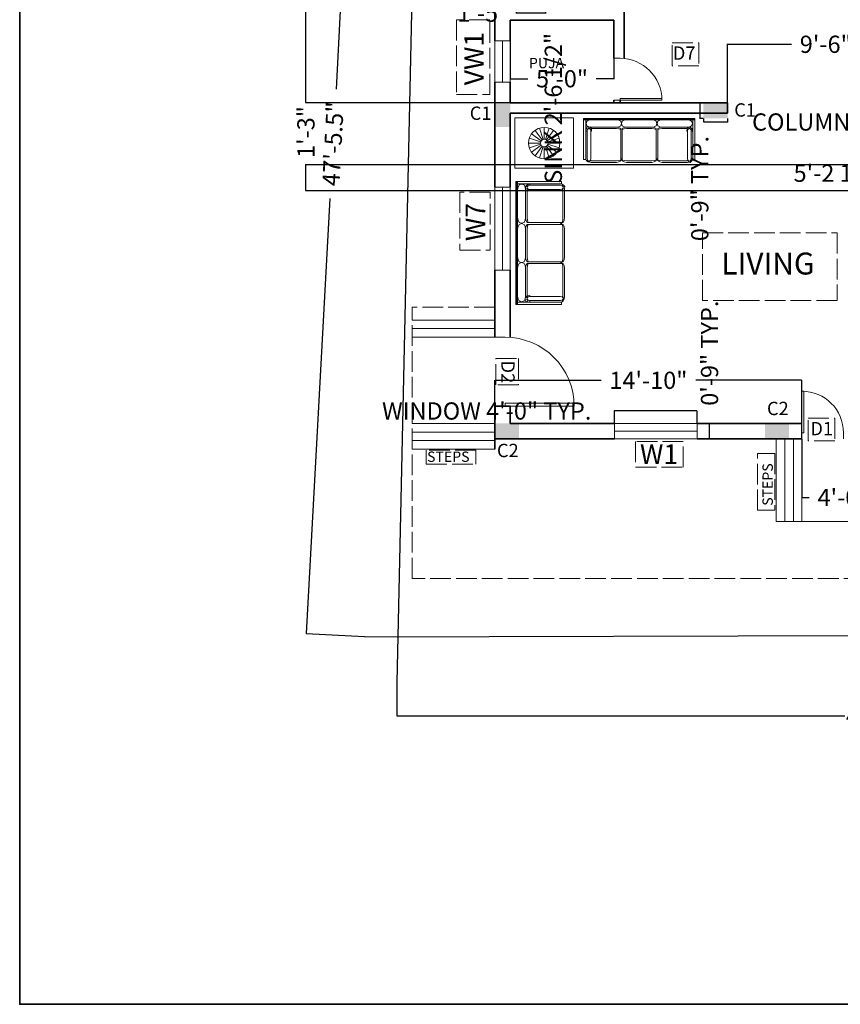
# Model space of a CAD drawing. Units: inches. Extents: x -269 to 4574, y -694 to 313.
# Tile 1 of 19: x -269 to 208, y -694 to -122. Entities that reach past the tile are written whole.
import ezdxf

# ---------------------------------------------------------------- set-up
doc = ezdxf.new("R2010")
doc.units = ezdxf.units.IN
doc.header["$MEASUREMENT"] = 0
doc.linetypes.add('ACAD_ISO02W100', pattern=[15, 12, -3])
for name, color, linetype, lineweight in [('A-ANNO-FRAM', 7, 'ACAD_ISO02W100', 13), ('A-ANNO-IDEN', 6, 'Continuous', 18), ('A-AREA-IDEN', 6, 'Continuous', 20), ('A-COLS', 5, 'Continuous', 35), ('A-COLS-IDEN', 6, 'Continuous', 18), ('A-FURN', 2, 'Continuous', 18), ('A-ROOF-OVHD', 1, 'ACAD_ISO02W100', 18), ('BORDER', 7, 'Continuous', 35), ('C-PROP', 7, 'Continuous', 25), ('DIMENSION', 5, 'Continuous', 18), ('DOORS', 3, 'Continuous', 18), ('STAIR', 4, 'Continuous', 20), ('TEXT', 6, 'Continuous', 18), ('WALL', 1, 'Continuous', 35), ('WINDOWS', 2, 'Continuous', 18)]:
    doc.layers.add(name, color=color, linetype=linetype, lineweight=lineweight)
doc.dimstyles.get("Standard").update_dxf_attribs({"dimtxt": 10, "dimasz": 0.18, "dimexe": 0.18, "dimexo": 0.0625, "dimgap": 0.09, "dimtad": 0, "dimdec": 1, "dimzin": 0, "dimdsep": 46, "dimlunit": 3, "dimtxsty": 'Standard', "dimcen": 0.09, "dimclrt": 7, "dimadec": 0, "dimazin": 0, "dimtfac": 1, "dimtdec": 1, "dimtofl": 0, "dimtmove": 0, "dimatfit": 3, "dimfxl": 1, "dimtolj": 1, "dimtzin": 0, "dimarcsym": 0})

# ---------------------------------------------------------------- blocks, each defined once
blk = doc.blocks.new('*U3')
for p, q in [((0, 0), (0, -6)), ((40, 0), (40, -6))]:
    blk.add_line(p, q)
blk.add_lwpolyline([(0, 0), (0, 40), (1.75, 40), (1.75, 0)], close=True)
blk.add_arc((0, 0), 40, 0, 90)
blk = doc.blocks.new('*D33')
at = {"layer": 'Defpoints', "color": 0, "lineweight": 0, "transparency": 16777216}
for p in [(-49.71, -506.83), (490.29, -506.83), (490.29, -526.5)]:
    blk.add_point(p, dxfattribs=at)
at = {"layer": 'DIMENSION', "color": 0, "lineweight": -2, "transparency": 16777216}
for p, q in [((-49.71, -506.9), (-49.71, -526.68)), ((490.29, -506.9), (490.29, -526.68)), ((-49.53, -526.5), (210.2, -526.5)), ((490.11, -526.5), (230.38, -526.5))]:
    blk.add_line(p, q, dxfattribs=at)
at = {"layer": 'DIMENSION', "color": 0, "lineweight": 0, "transparency": 16777216}
for points in [[(-49.53, -526.47), (-49.53, -526.53), (-49.71, -526.5)], [(490.11, -526.47), (490.11, -526.53), (490.29, -526.5)]]:
    blk.add_solid(points, dxfattribs=at)
at = {"layer": 'DIMENSION', "color": 0, "transparency": 16777216, "insert": (220.29, -526.5), "char_height": 10, "attachment_point": 5}
blk.add_mtext("\\A1;45'", dxfattribs=at)
blk = doc.blocks.new('*D34')
at = {"layer": 'Defpoints', "color": 0, "lineweight": 0, "transparency": 16777216}
for p in [(-37.71, 88), (-102.08, -478.85), (-68.45, -480.67)]:
    blk.add_point(p, dxfattribs=at)
at = {"layer": 'DIMENSION', "color": 0, "lineweight": -2, "transparency": 16777216}
for p, q in [((-71.35, 89.64), (-85, -162.81)), ((-37.77, 88), (-71.52, 89.83)), ((-102.07, -478.67), (-88.43, -226.23)), ((-68.51, -480.67), (-102.26, -478.84))]:
    blk.add_line(p, q, dxfattribs=at)
at = {"layer": 'DIMENSION', "color": 0, "lineweight": 0, "transparency": 16777216}
for points in [[(-71.38, 89.64), (-71.32, 89.64), (-71.34, 89.82)], [(-102.1, -478.67), (-102.04, -478.67), (-102.08, -478.85)]]:
    blk.add_solid(points, dxfattribs=at)
at = {"layer": 'DIMENSION', "color": 0, "transparency": 16777216, "insert": (-86.71, -194.52), "char_height": 10, "attachment_point": 5, "rotation": 86.9054}
blk.add_mtext('\\A1;47\'-5.5"', dxfattribs=at)
blk = doc.blocks.new('GLAZ-48IN')
blk.add_line((4.5, 0), (4.5, 48))
blk.add_lwpolyline([(0, 48), (9, 48), (9, 0), (0, 0)], close=True)
blk = doc.blocks.new('GLAZ-24IN')
blk.add_line((4.5, 24), (4.5, 0))
blk.add_lwpolyline([(0, 24), (9, 24), (9, 0), (0, 0)], close=True)
blk = doc.blocks.new('TAG-DOOR-FRAME')
blk.add_lwpolyline([(0, 13.18), (15.39, 13.18), (15.39, 0), (0, 0)], close=True)
blk = doc.blocks.new('COLUMN-9x14-PLAN')
h = blk.add_hatch(color=256)
h.dxf.hatch_style = 1
h.paths.add_polyline_path([(9, 14), (0, 14), (0, 0), (9, 0), (9, 5)])
blk = doc.blocks.new('*D50')
at = {"layer": 'Defpoints', "color": 0, "lineweight": 0, "transparency": 16777216}
for p in [(281.85, -211.53), (281.85, -221.79), (344.28, -221.79)]:
    blk.add_point(p, dxfattribs=at)
at = {"layer": 'DIMENSION', "color": 0, "lineweight": -2, "transparency": 16777216}
for p, q in [((281.85, -221.73), (281.85, -211.35)), ((344.28, -221.73), (344.28, -211.35)), ((281.85, -211.53), (281.67, -211.53)), ((344.1, -211.53), (282.03, -211.53))]:
    blk.add_line(p, q, dxfattribs=at)
at = {"layer": 'DIMENSION', "color": 0, "lineweight": 0, "transparency": 16777216}
for points in [[(282.03, -211.5), (282.03, -211.56), (281.85, -211.53)], [(344.1, -211.5), (344.1, -211.56), (344.28, -211.53)]]:
    blk.add_solid(points, dxfattribs=at)
at = {"layer": 'DIMENSION', "color": 7, "transparency": 16777216, "insert": (222.77, -211.53), "char_height": 10, "attachment_point": 5}
blk.add_mtext('\\A1;5\'-2 1/2" TYP.', dxfattribs=at)
blk = doc.blocks.new('*D51')
at = {"layer": 'Defpoints', "color": 0, "lineweight": 0, "transparency": 16777216}
for p in [(128.14, -179.73), (142.14, -179.73), (142.14, -181.83)]:
    blk.add_point(p, dxfattribs=at)
at = {"layer": 'DIMENSION', "color": 0, "lineweight": -2, "transparency": 16777216}
for p, q in [((128.14, -179.79), (128.14, -182.01)), ((128.32, -181.83), (141.96, -181.83)), ((142.14, -179.79), (142.14, -182.01)), ((142.14, -181.83), (142.32, -181.83))]:
    blk.add_line(p, q, dxfattribs=at)
at = {"layer": 'DIMENSION', "color": 0, "lineweight": 0, "transparency": 16777216}
for points in [[(128.32, -181.8), (128.32, -181.86), (128.14, -181.83)], [(141.96, -181.8), (141.96, -181.86), (142.14, -181.83)]]:
    blk.add_solid(points, dxfattribs=at)
at = {"layer": 'DIMENSION', "color": 7, "transparency": 16777216, "insert": (216.93, -181.83), "char_height": 10, "attachment_point": 5}
blk.add_mtext('\\A1;COLUMN 1\'-2" TYP.', dxfattribs=at)
blk = doc.blocks.new('*D52')
at = {"layer": 'Defpoints', "color": 0, "lineweight": 0, "transparency": 16777216}
for p in [(128.14, -170.73), (126.04, -179.73), (128.14, -179.73)]:
    blk.add_point(p, dxfattribs=at)
at = {"layer": 'DIMENSION', "color": 0, "lineweight": -2, "transparency": 16777216}
for p, q in [((128.08, -170.73), (125.86, -170.73)), ((126.04, -170.91), (126.04, -179.55)), ((128.08, -179.73), (125.86, -179.73)), ((126.04, -179.73), (126.04, -179.91))]:
    blk.add_line(p, q, dxfattribs=at)
at = {"layer": 'DIMENSION', "color": 0, "lineweight": 0, "transparency": 16777216}
for points in [[(126.01, -170.91), (126.07, -170.91), (126.04, -170.73)], [(126.01, -179.55), (126.07, -179.55), (126.04, -179.73)]]:
    blk.add_solid(points, dxfattribs=at)
at = {"layer": 'DIMENSION', "color": 7, "transparency": 16777216, "insert": (126.04, -220.47), "char_height": 10, "attachment_point": 5, "rotation": 90}
blk.add_mtext('\\A1;0\'-9" TYP.', dxfattribs=at)
blk = doc.blocks.new('*D53')
at = {"layer": 'Defpoints', "color": 0, "lineweight": 0, "transparency": 16777216}
for p in [(76.5, -349.53), (76.5, -356.73), (124.5, -356.73)]:
    blk.add_point(p, dxfattribs=at)
at = {"layer": 'DIMENSION', "color": 0, "lineweight": -2, "transparency": 16777216}
for p, q in [((76.5, -349.53), (76.32, -349.53)), ((76.5, -356.67), (76.5, -349.35)), ((124.32, -349.53), (76.68, -349.53)), ((124.5, -356.67), (124.5, -349.35))]:
    blk.add_line(p, q, dxfattribs=at)
at = {"layer": 'DIMENSION', "color": 0, "lineweight": 0, "transparency": 16777216}
for points in [[(76.68, -349.5), (76.68, -349.56), (76.5, -349.53)], [(124.32, -349.5), (124.32, -349.56), (124.5, -349.53)]]:
    blk.add_solid(points, dxfattribs=at)
at = {"layer": 'DIMENSION', "color": 7, "transparency": 16777216, "insert": (2.42, -349.53), "char_height": 10, "attachment_point": 5}
blk.add_mtext('\\A1;WINDOW 4\'-0" TYP.', dxfattribs=at)
blk = doc.blocks.new('*D54')
at = {"layer": 'Defpoints', "color": 0, "lineweight": 0, "transparency": 16777216}
for p in [(124.5, -356.73), (131.7, -356.73), (124.5, -365.73)]:
    blk.add_point(p, dxfattribs=at)
at = {"layer": 'DIMENSION', "color": 0, "lineweight": -2, "transparency": 16777216}
for p, q in [((124.56, -356.73), (131.88, -356.73)), ((131.7, -356.73), (131.7, -356.55)), ((131.7, -365.55), (131.7, -356.91)), ((124.56, -365.73), (131.88, -365.73))]:
    blk.add_line(p, q, dxfattribs=at)
at = {"layer": 'DIMENSION', "color": 0, "lineweight": 0, "transparency": 16777216}
for points in [[(131.67, -356.91), (131.73, -356.91), (131.7, -356.73)], [(131.67, -365.55), (131.73, -365.55), (131.7, -365.73)]]:
    blk.add_solid(points, dxfattribs=at)
at = {"layer": 'DIMENSION', "color": 7, "transparency": 16777216, "insert": (131.7, -315.99), "char_height": 10, "attachment_point": 5, "rotation": 90}
blk.add_mtext('\\A1;0\'-9" TYP.', dxfattribs=at)
blk = doc.blocks.new('*D61')
at = {"layer": 'Defpoints', "color": 0, "lineweight": 0, "transparency": 16777216}
for p in [(36.5, -83.55), (36.5, -114.1), (41.08, -114.1)]:
    blk.add_point(p, dxfattribs=at)
at = {"layer": 'DIMENSION', "color": 0, "lineweight": -2, "transparency": 16777216}
for p, q in [((36.56, -83.55), (41.26, -83.55)), ((41.08, -83.73), (41.08, -113.92)), ((36.56, -114.1), (41.26, -114.1)), ((41.08, -114.1), (41.08, -114.28))]:
    blk.add_line(p, q, dxfattribs=at)
at = {"layer": 'DIMENSION', "color": 0, "lineweight": 0, "transparency": 16777216}
for points in [[(41.05, -83.73), (41.11, -83.73), (41.08, -83.55)], [(41.05, -113.92), (41.11, -113.92), (41.08, -114.1)]]:
    blk.add_solid(points, dxfattribs=at)
at = {"layer": 'DIMENSION', "color": 7, "transparency": 16777216, "insert": (41.08, -173.89), "char_height": 10, "attachment_point": 5, "rotation": 90}
blk.add_mtext('\\A1;SINK 2\'-6 1/2"', dxfattribs=at)
blk = doc.blocks.new('*D62')
at = {"layer": 'Defpoints', "color": 0, "lineweight": 0, "transparency": 16777216}
for p in [(19.53, -114.1), (36.5, -114.1), (19.53, -118.68)]:
    blk.add_point(p, dxfattribs=at)
at = {"layer": 'DIMENSION', "color": 0, "lineweight": -2, "transparency": 16777216}
for p, q in [((19.53, -114.16), (19.53, -118.86)), ((36.5, -114.16), (36.5, -118.86)), ((19.53, -118.68), (19.35, -118.68)), ((36.32, -118.68), (19.71, -118.68))]:
    blk.add_line(p, q, dxfattribs=at)
at = {"layer": 'DIMENSION', "color": 0, "lineweight": 0, "transparency": 16777216}
for points in [[(19.71, -118.65), (19.71, -118.71), (19.53, -118.68)], [(36.32, -118.65), (36.32, -118.71), (36.5, -118.68)]]:
    blk.add_solid(points, dxfattribs=at)
at = {"layer": 'DIMENSION', "color": 7, "transparency": 16777216, "insert": (0.45, -118.68), "char_height": 10, "attachment_point": 5}
blk.add_mtext('\\A1;1\'-5"', dxfattribs=at)
blk = doc.blocks.new('*D76')
at = {"layer": 'Defpoints', "color": 0, "lineweight": 0, "transparency": 16777216}
for p in [(7.14, 18.27), (-102.45, -170.73), (16.14, -170.73)]:
    blk.add_point(p, dxfattribs=at)
at = {"layer": 'DIMENSION', "color": 0, "lineweight": -2, "transparency": 16777216}
for p, q in [((7.07, 18.27), (-102.63, 18.27)), ((-102.45, 18.09), (-102.45, -52.57)), ((-102.45, -170.55), (-102.45, -99.89)), ((16.07, -170.73), (-102.63, -170.73))]:
    blk.add_line(p, q, dxfattribs=at)
at = {"layer": 'DIMENSION', "color": 0, "lineweight": 0, "transparency": 16777216}
for points in [[(-102.48, 18.09), (-102.42, 18.09), (-102.45, 18.27)], [(-102.48, -170.55), (-102.42, -170.55), (-102.45, -170.73)]]:
    blk.add_solid(points, dxfattribs=at)
at = {"layer": 'DIMENSION', "color": 7, "transparency": 16777216, "insert": (-102.45, -76.23), "char_height": 10, "attachment_point": 5, "rotation": 90}
blk.add_mtext('\\A1;15\'-9"', dxfattribs=at)
blk = doc.blocks.new('*D77')
at = {"layer": 'Defpoints', "color": 0, "lineweight": 0, "transparency": 16777216}
for p in [(256.14, -136.73), (142.14, -170.73), (256.14, -170.73)]:
    blk.add_point(p, dxfattribs=at)
at = {"layer": 'DIMENSION', "color": 0, "lineweight": -2, "transparency": 16777216}
for p, q in [((142.14, -170.67), (142.14, -136.55)), ((142.32, -136.73), (179.29, -136.73)), ((255.96, -136.73), (218.99, -136.73)), ((256.14, -170.67), (256.14, -136.55))]:
    blk.add_line(p, q, dxfattribs=at)
at = {"layer": 'DIMENSION', "color": 0, "lineweight": 0, "transparency": 16777216}
for points in [[(142.32, -136.7), (142.32, -136.76), (142.14, -136.73)], [(255.96, -136.7), (255.96, -136.76), (256.14, -136.73)]]:
    blk.add_solid(points, dxfattribs=at)
at = {"layer": 'DIMENSION', "color": 7, "transparency": 16777216, "insert": (199.14, -136.73), "char_height": 10, "attachment_point": 5}
blk.add_mtext('\\A1;9\'-6"', dxfattribs=at)
blk = doc.blocks.new('*D78')
at = {"layer": 'Defpoints', "color": 0, "lineweight": 0, "transparency": 16777216}
for p in [(185.34, -331.73), (7.14, -365.73), (185.34, -365.73)]:
    blk.add_point(p, dxfattribs=at)
at = {"layer": 'DIMENSION', "color": 0, "lineweight": -2, "transparency": 16777216}
for p, q in [((7.14, -365.67), (7.14, -331.55)), ((7.32, -331.73), (68.77, -331.73)), ((185.16, -331.73), (123.71, -331.73)), ((185.34, -365.67), (185.34, -331.55))]:
    blk.add_line(p, q, dxfattribs=at)
at = {"layer": 'DIMENSION', "color": 0, "lineweight": 0, "transparency": 16777216}
for points in [[(7.32, -331.7), (7.32, -331.76), (7.14, -331.73)], [(185.16, -331.7), (185.16, -331.76), (185.34, -331.73)]]:
    blk.add_solid(points, dxfattribs=at)
at = {"layer": 'DIMENSION', "color": 7, "transparency": 16777216, "insert": (96.24, -331.73), "char_height": 10, "attachment_point": 5}
blk.add_mtext('\\A1;14\'-10"', dxfattribs=at)
blk = doc.blocks.new('*D79')
at = {"layer": 'Defpoints', "color": 0, "lineweight": 0, "transparency": 16777216}
for p in [(185.34, -365.73), (233.52, -365.73), (185.34, -399.73)]:
    blk.add_point(p, dxfattribs=at)
at = {"layer": 'DIMENSION', "color": 0, "lineweight": -2, "transparency": 16777216}
for p, q in [((185.34, -365.79), (185.34, -399.91)), ((233.52, -365.79), (233.52, -399.91)), ((185.52, -399.73), (189.58, -399.73)), ((233.34, -399.73), (229.29, -399.73))]:
    blk.add_line(p, q, dxfattribs=at)
at = {"layer": 'DIMENSION', "color": 0, "lineweight": 0, "transparency": 16777216}
for points in [[(185.52, -399.7), (185.52, -399.76), (185.34, -399.73)], [(233.34, -399.7), (233.34, -399.76), (233.52, -399.73)]]:
    blk.add_solid(points, dxfattribs=at)
at = {"layer": 'DIMENSION', "color": 7, "transparency": 16777216, "insert": (209.43, -399.73), "char_height": 10, "attachment_point": 5}
blk.add_mtext('\\A1;4\'-0"', dxfattribs=at)
blk = doc.blocks.new('*D81')
at = {"layer": 'Defpoints', "color": 0, "lineweight": 0, "transparency": 16777216}
for p in [(-102.45, -206.73), (262.14, -206.73), (266.7, -221.79)]:
    blk.add_point(p, dxfattribs=at)
at = {"layer": 'DIMENSION', "color": 0, "lineweight": -2, "transparency": 16777216}
for p, q in [((262.07, -206.73), (-102.63, -206.73)), ((-102.45, -206.73), (-102.45, -206.55)), ((-102.45, -221.61), (-102.45, -206.91)), ((266.64, -221.79), (-102.63, -221.79))]:
    blk.add_line(p, q, dxfattribs=at)
at = {"layer": 'DIMENSION', "color": 0, "lineweight": 0, "transparency": 16777216}
for points in [[(-102.48, -206.91), (-102.42, -206.91), (-102.45, -206.73)], [(-102.48, -221.61), (-102.42, -221.61), (-102.45, -221.79)]]:
    blk.add_solid(points, dxfattribs=at)
at = {"layer": 'DIMENSION', "color": 7, "transparency": 16777216, "insert": (-102.45, -187.65), "char_height": 10, "attachment_point": 5, "rotation": 90}
blk.add_mtext('\\A1;1\'-3"', dxfattribs=at)
blk = doc.blocks.new('*D83')
at = {"layer": 'Defpoints', "color": 0, "lineweight": 0, "transparency": 16777216}
for p in [(16.14, -122.73), (76.14, -122.73), (16.14, -156.73)]:
    blk.add_point(p, dxfattribs=at)
at = {"layer": 'DIMENSION', "color": 0, "lineweight": -2, "transparency": 16777216}
for p, q in [((16.14, -122.79), (16.14, -156.91)), ((76.14, -122.79), (76.14, -156.91)), ((16.32, -156.73), (26.29, -156.73)), ((75.96, -156.73), (65.99, -156.73))]:
    blk.add_line(p, q, dxfattribs=at)
at = {"layer": 'DIMENSION', "color": 0, "lineweight": 0, "transparency": 16777216}
for points in [[(16.32, -156.7), (16.32, -156.76), (16.14, -156.73)], [(75.96, -156.7), (75.96, -156.76), (76.14, -156.73)]]:
    blk.add_solid(points, dxfattribs=at)
at = {"layer": 'DIMENSION', "color": 7, "transparency": 16777216, "insert": (46.14, -156.73), "char_height": 10, "attachment_point": 5}
blk.add_mtext('\\A1;5\'-0"', dxfattribs=at)

msp = doc.modelspace()

# ---------------------------------------------------------------- linework, layer by layer
at = {"layer": 'A-ANNO-FRAM'}
for points in [[(4.33, -122.49), (-15.09, -122.49), (-15.09, -165.87), (4.33, -165.87)], [(4.45, -222.47), (-13.15, -222.47), (-13.15, -256.24), (4.45, -256.24)], [(127.57, -246.18), (205.73, -246.18), (205.73, -285.44), (127.57, -285.44)], [(116.44, -367.26), (88.85, -367.26), (88.85, -382.1), (116.44, -382.1)], [(-3.91, -372.33), (-32.62, -372.33), (-32.62, -380.48), (-3.91, -380.48)], [(159.51, -374.12), (169.58, -374.12), (169.58, -407.14), (159.51, -407.14)], [(91.35, -380.23), (91.35, -380.23), (91.35, -380.23), (91.35, -380.23)]]:
    msp.add_lwpolyline(points, close=True, dxfattribs=at)
at = {"layer": 'A-FURN'}
for p, q in [((58.62, -179.77), (58.62, -179.76)), ((58.62, -179.76), (58.62, -203.68)), ((123.2, -179.76), (58.62, -179.76)), ((59.87, -179.77), (58.62, -179.77)), ((58.62, -179.81), (59.87, -179.81)), ((59.87, -179.86), (58.62, -179.86)), ((58.62, -179.94), (59.87, -179.94)), ((59.87, -180.03), (58.62, -180.03)), ((58.62, -180.12), (123.2, -180.12)), ((59.87, -180.23), (58.62, -180.23)), ((58.62, -180.36), (59.87, -180.36)), ((58.62, -180.48), (123.2, -180.48)), ((59.87, -203.68), (59.87, -179.76)), ((59.87, -180.19), (121.95, -180.19)), ((121.95, -180.25), (59.87, -180.25)), ((59.87, -180.3), (121.95, -180.3)), ((121.95, -180.35), (59.87, -180.35)), ((59.87, -180.39), (121.95, -180.39)), ((121.95, -180.43), (59.87, -180.43)), ((121.95, -180.46), (59.87, -180.46)), ((59.87, -180.46), (59.87, -180.47)), ((59.87, -180.47), (121.95, -180.47)), ((60.07, -182.71), (60.54, -181.35)), ((60.54, -181.61), (60.07, -182.71)), ((60.54, -184.07), (60.07, -182.71)), ((61.65, -180.83), (60.54, -181.35)), ((63.01, -180.61), (61.65, -180.83)), ((77.68, -180.61), (63.01, -180.61)), ((79.05, -180.83), (77.68, -180.61)), ((80.16, -181.35), (79.05, -180.83)), ((80.59, -182.63), (80.16, -181.35)), ((80.16, -184.07), (80.59, -182.78)), ((80.59, -182.62), (81.03, -181.35)), ((81.03, -184.06), (80.59, -182.79)), ((82.14, -180.83), (81.03, -181.35)), ((83.5, -180.61), (82.14, -180.83)), ((98.18, -180.61), (83.5, -180.61)), ((99.55, -180.83), (98.18, -180.61)), ((100.66, -181.35), (99.55, -180.83)), ((100.66, -181.35), (101.12, -182.71)), ((100.66, -184.06), (101.12, -182.71)), ((101.25, -182.71), (101.71, -181.35)), ((101.71, -184.06), (101.25, -182.71)), ((101.71, -181.35), (102.83, -180.83)), ((102.83, -180.83), (104.19, -180.61)), ((104.19, -180.61), (118.87, -180.61)), ((118.87, -180.61), (120.23, -180.83)), ((120.23, -180.83), (121.34, -181.35)), ((121.34, -181.35), (121.81, -182.71)), ((121.34, -184.06), (121.81, -182.71)), ((121.95, -179.77), (121.95, -179.76)), ((121.95, -179.76), (121.95, -203.68)), ((123.2, -179.77), (121.95, -179.77)), ((121.95, -179.81), (123.2, -179.81)), ((123.2, -179.86), (121.95, -179.86)), ((121.95, -179.94), (123.2, -179.94)), ((123.2, -180.03), (121.95, -180.03)), ((121.95, -180.23), (123.2, -180.23)), ((123.2, -180.36), (121.95, -180.36)), ((123.2, -203.68), (123.2, -179.76)), ((34.54, -192.26), (30.48, -186.68)), ((35.15, -191.95), (33.02, -185.39)), ((35.83, -191.84), (35.83, -184.94)), ((36.5, -191.95), (38.63, -185.39)), ((37.11, -192.26), (41.17, -186.68)), ((58.61, -200.13), (58.61, -183.39)), ((58.61, -183.39), (58.62, -183.39)), ((61.17, -184.36), (59.87, -185.04)), ((60.89, -186.12), (59.87, -185.04)), ((59.87, -185.04), (59.87, -187.02)), ((59.87, -187.02), (60.68, -187.02)), ((60.68, -187.06), (59.87, -187.06)), ((60.08, -187.03), (60.07, -187.04)), ((60.07, -187.04), (60.08, -187.04)), ((60.08, -187.06), (60.08, -187.02)), ((60.26, -187.02), (60.26, -187.06)), ((60.68, -187.05), (60.26, -187.06)), ((60.54, -184.07), (61.65, -184.58)), ((60.89, -186.12), (60.68, -187.03)), ((60.68, -187.03), (60.68, -203.04)), ((61.43, -185.57), (60.89, -186.12)), ((61.43, -185.57), (61.17, -184.36)), ((62.11, -185.57), (61.43, -185.57)), ((61.65, -184.58), (63.01, -184.81)), ((62.11, -185.57), (62.24, -185.01)), ((62.64, -186.14), (62.11, -185.57)), ((62.24, -185.01), (62.31, -184.69)), ((63.17, -185.61), (62.33, -184.7)), ((62.64, -186.14), (63.17, -185.61)), ((62.85, -187.05), (62.64, -186.14)), ((62.81, -184.78), (62.83, -184.78)), ((62.85, -203.02), (62.85, -187.05)), ((62.85, -187.05), (63.26, -187.06)), ((63.01, -184.81), (77.68, -184.81)), ((63.1, -185.61), (77.68, -185.61)), ((63.26, -187.06), (63.17, -185.61)), ((77.68, -184.81), (79.05, -184.58)), ((77.68, -185.61), (79.05, -185.77)), ((79.05, -185), (77.86, -184.78)), ((79.05, -184.58), (80.16, -184.07)), ((80.16, -185.57), (79.05, -185)), ((79.05, -185.77), (80.16, -186.12)), ((80.16, -204.46), (80.16, -185.57)), ((81.03, -184.06), (82.14, -184.58)), ((81.03, -185.57), (82.14, -184.99)), ((81.03, -185.57), (81.03, -204.46)), ((81.03, -186.12), (82.14, -185.77)), ((82.14, -184.58), (83.5, -184.8)), ((82.14, -184.99), (83.34, -184.78)), ((82.14, -185.77), (83.5, -185.61)), ((83.5, -184.8), (98.18, -184.8)), ((83.5, -185.61), (98.18, -185.61)), ((98.18, -184.8), (99.55, -184.58)), ((98.18, -185.61), (99.55, -185.77)), ((98.34, -184.78), (99.55, -184.99)), ((99.55, -184.58), (100.66, -184.06)), ((99.55, -184.99), (100.66, -185.57)), ((99.55, -185.77), (100.66, -186.12)), ((100.66, -185.57), (100.66, -204.46)), ((102.83, -184.58), (101.71, -184.06)), ((101.71, -185.57), (102.83, -184.99)), ((101.71, -185.57), (101.71, -204.46)), ((102.83, -185.77), (101.71, -186.12)), ((104.19, -184.8), (102.83, -184.58)), ((102.83, -184.99), (104.03, -184.78)), ((104.19, -185.61), (102.83, -185.77)), ((118.87, -184.8), (104.19, -184.8)), ((118.71, -185.61), (104.19, -185.61)), ((118.54, -187.06), (118.65, -185.61)), ((118.54, -187.06), (118.96, -187.05)), ((118.65, -185.61), (119.03, -184.78)), ((118.65, -185.61), (119.16, -186.14)), ((120.23, -184.58), (118.87, -184.8)), ((119.16, -186.14), (118.96, -187.05)), ((118.96, -187.05), (118.96, -203.02)), ((119.03, -184.78), (119.51, -184.76)), ((119.7, -185.57), (119.16, -186.14)), ((119.51, -184.76), (120.56, -184.75)), ((119.51, -184.76), (119.7, -185.57)), ((119.7, -185.57), (120.38, -185.57)), ((121.34, -184.06), (120.23, -184.58)), ((120.38, -185.57), (120.56, -184.75)), ((120.92, -186.12), (120.38, -185.57)), ((120.56, -184.75), (121.41, -185.61)), ((120.92, -186.12), (121.41, -185.61)), ((121.14, -187.03), (120.92, -186.12)), ((121.14, -187.03), (121.56, -187.02)), ((121.14, -203.04), (121.14, -187.03)), ((121.56, -187.06), (121.14, -187.05)), ((121.41, -185.61), (121.81, -187.04)), ((121.56, -187.02), (121.74, -187.02)), ((121.56, -187.02), (121.56, -187.06)), ((121.74, -187.06), (121.56, -187.06)), ((121.74, -187.02), (121.74, -187.06)), ((121.81, -187.04), (121.74, -187.03)), ((121.74, -187.04), (121.81, -187.04)), ((123.21, -183.39), (123.2, -183.39)), ((123.21, -200.13), (123.21, -183.39)), ((33.64, -194.03), (26.74, -194.03)), ((33.74, -193.36), (27.18, -191.22)), ((34.05, -192.74), (28.47, -188.69)), ((37.6, -192.74), (43.18, -188.69)), ((37.91, -193.36), (44.47, -191.22)), ((38.02, -194.03), (44.91, -194.03)), ((33.74, -194.71), (27.18, -196.84)), ((34.05, -195.32), (28.47, -199.37)), ((34.54, -195.8), (30.48, -201.38)), ((35.15, -196.12), (33.02, -202.68)), ((35.83, -196.22), (35.83, -203.12)), ((36.5, -196.12), (38.63, -202.68)), ((37.11, -195.8), (41.17, -201.38)), ((37.6, -195.32), (43.18, -199.37)), ((37.91, -194.71), (44.47, -196.84)), ((58.62, -200.13), (58.61, -200.13)), ((59.87, -203.66), (58.62, -203.66)), ((59.87, -203.67), (59.87, -203.66)), ((60.41, -204.46), (59.87, -203.68)), ((60.41, -204.46), (60.55, -204.3)), ((60.41, -204.46), (61.33, -204.97)), ((60.55, -204.3), (60.89, -203.95)), ((60.68, -203.04), (60.89, -203.95)), ((60.89, -203.95), (61.43, -204.5)), ((61.43, -204.5), (61.33, -204.97)), ((63.01, -205.28), (61.33, -204.97)), ((61.43, -204.5), (62.11, -204.49)), ((62.11, -204.49), (62.64, -203.93)), ((62.26, -205.14), (62.11, -204.49)), ((62.85, -203.02), (62.64, -203.93)), ((62.64, -203.93), (62.99, -204.27)), ((62.99, -204.27), (63.14, -204.42)), ((77.68, -205.28), (63.01, -205.28)), ((63.14, -204.41), (77.68, -204.41)), ((77.68, -204.41), (79.05, -204.26)), ((79.05, -205.03), (77.68, -205.28)), ((79.05, -204.26), (80.16, -203.91)), ((80.16, -204.46), (79.05, -205.03)), ((80.59, -203.08), (80.16, -204.46)), ((80.4, -203.68), (80.41, -203.67)), ((80.78, -203.68), (80.4, -203.68)), ((80.41, -203.67), (80.77, -203.67)), ((80.77, -203.63), (80.42, -203.63)), ((80.44, -203.58), (80.75, -203.58)), ((80.59, -203.08), (81.03, -204.46)), ((81.03, -203.9), (82.14, -204.26)), ((82.14, -205.03), (81.03, -204.46)), ((82.14, -204.26), (83.5, -204.41)), ((83.5, -205.28), (82.14, -205.03)), ((83.5, -204.41), (98.18, -204.41)), ((98.18, -205.28), (83.5, -205.28)), ((98.18, -204.41), (99.55, -204.26)), ((99.55, -205.03), (98.18, -205.28)), ((99.55, -204.26), (100.66, -203.9)), ((100.66, -204.46), (99.55, -205.03)), ((101.25, -202.99), (100.66, -204.46)), ((100.97, -203.67), (101.46, -203.67)), ((101.47, -203.68), (100.97, -203.68)), ((101.25, -202.99), (101.71, -204.46)), ((102.83, -204.26), (101.71, -203.9)), ((101.71, -204.46), (102.83, -205.03)), ((104.19, -204.41), (102.83, -204.26)), ((102.83, -205.03), (104.19, -205.28)), ((118.67, -204.41), (104.19, -204.41)), ((104.19, -205.28), (118.87, -205.28)), ((118.68, -204.42), (118.83, -204.27)), ((118.83, -204.27), (119.16, -203.93)), ((118.87, -205.28), (119.39, -205.18)), ((118.96, -203.02), (119.16, -203.93)), ((119.16, -203.93), (119.7, -204.49)), ((119.39, -205.18), (120.56, -205.32)), ((119.54, -205.2), (119.7, -204.49)), ((119.7, -204.49), (120.38, -204.5)), ((120.38, -204.5), (120.92, -203.95)), ((120.38, -204.5), (120.56, -205.32)), ((120.56, -205.32), (121.41, -204.46)), ((121.14, -203.04), (120.92, -203.95)), ((120.92, -203.95), (121.41, -204.46)), ((121.41, -204.46), (121.95, -203.68)), ((121.95, -203.68), (121.95, -203.66)), ((121.95, -203.66), (123.2, -203.66)), ((123.2, -200.13), (123.21, -200.13)), ((123.2, -203.66), (123.2, -203.68)), ((45.87, -216.29), (19.42, -216.29)), ((19.42, -216.29), (19.42, -287.73)), ((19.43, -216.29), (19.43, -217.68)), ((19.47, -217.68), (19.47, -216.29)), ((19.53, -216.29), (19.53, -217.68)), ((19.61, -217.68), (19.61, -216.29)), ((19.71, -216.29), (19.71, -217.68)), ((19.82, -287.73), (19.82, -216.29)), ((19.94, -217.68), (19.94, -216.29)), ((20.08, -216.29), (20.08, -217.68)), ((20.22, -287.73), (20.22, -216.29)), ((41.95, -216.28), (23.44, -216.28)), ((23.44, -216.28), (23.44, -216.29)), ((41.95, -216.29), (41.95, -216.28)), ((45.85, -217.68), (45.85, -216.29)), ((45.85, -216.29), (45.87, -216.29)), ((19.43, -217.68), (19.42, -217.68)), ((19.42, -217.68), (45.87, -217.68)), ((19.89, -286.35), (19.89, -217.68)), ((19.96, -217.68), (19.96, -286.35)), ((20.02, -286.35), (20.02, -217.68)), ((20.07, -217.68), (20.07, -286.35)), ((20.12, -286.35), (20.12, -217.68)), ((20.16, -217.68), (20.16, -286.35)), ((20.19, -217.68), (20.19, -286.35)), ((20.21, -286.35), (20.21, -217.68)), ((20.35, -221.08), (20.6, -219.58)), ((20.35, -237.32), (20.35, -221.08)), ((20.6, -219.58), (21.18, -218.35)), ((21.18, -218.35), (22.68, -217.83)), ((24.17, -218.35), (22.68, -217.83)), ((24.17, -218.35), (24.75, -219.58)), ((24.75, -219.58), (25, -221.08)), ((24.94, -219.21), (25.89, -218.27)), ((25.84, -219.41), (24.94, -219.21)), ((24.95, -220.37), (24.94, -219.21)), ((24.95, -220.37), (25.84, -220.16)), ((24.97, -220.91), (24.95, -220.37)), ((25.89, -221.32), (24.97, -220.91)), ((25, -221.08), (25, -237.32)), ((26.46, -218.81), (25.84, -219.41)), ((25.84, -220.16), (25.84, -219.41)), ((25.84, -220.16), (26.48, -220.75)), ((25.89, -218.27), (27.47, -217.83)), ((26.46, -218.81), (25.89, -218.27)), ((25.89, -221.32), (26.48, -220.75)), ((25.89, -221.25), (25.89, -237.32)), ((27.49, -221.44), (25.89, -221.32)), ((27.46, -218.57), (26.46, -218.81)), ((26.48, -220.75), (27.48, -220.98)), ((27.45, -218.11), (27.45, -217.91)), ((27.45, -217.91), (27.49, -217.91)), ((27.46, -218.57), (27.45, -218.11)), ((27.45, -218.11), (27.49, -218.11)), ((27.47, -217.83), (27.46, -217.91)), ((45.17, -218.57), (27.46, -218.57)), ((27.47, -217.91), (27.47, -217.83)), ((27.49, -218.11), (27.48, -218.57)), ((27.48, -220.98), (45.15, -220.98)), ((27.49, -221.44), (27.48, -220.98)), ((27.49, -217.91), (27.49, -218.11)), ((45.15, -220.98), (46.15, -220.75)), ((45.17, -218.57), (46.17, -218.81)), ((45.87, -217.68), (45.85, -217.68)), ((46.74, -218.27), (45.87, -217.68)), ((46.15, -220.75), (46.78, -220.16)), ((46.53, -221.13), (46.15, -220.75)), ((46.17, -218.81), (46.74, -218.27)), ((46.79, -219.41), (46.17, -218.81)), ((46.7, -221.29), (46.53, -221.13)), ((46.69, -221.3), (46.69, -237.32)), ((47.69, -219.21), (46.74, -218.27)), ((46.78, -220.16), (46.79, -219.41)), ((47.55, -220.34), (46.78, -220.16)), ((46.79, -219.41), (47.69, -219.21)), ((47.53, -220.5), (47.69, -219.21)), ((47.64, -221.08), (47.53, -220.5)), ((47.64, -237.32), (47.64, -221.08)), ((20.6, -238.83), (20.35, -237.32)), ((21.18, -240.06), (20.6, -238.83)), ((24.75, -238.83), (24.17, -240.06)), ((25, -237.32), (24.75, -238.83)), ((25.2, -238.83), (24.97, -237.5)), ((25.84, -240.06), (25.2, -238.83)), ((25.89, -237.32), (26.06, -238.83)), ((26.06, -238.83), (26.46, -240.06)), ((46.52, -238.83), (46.12, -240.06)), ((46.69, -237.32), (46.52, -238.83)), ((46.74, -240.06), (47.37, -238.83)), ((47.37, -238.83), (47.64, -237.32)), ((20.6, -242.46), (20.35, -243.96)), ((20.35, -243.96), (20.35, -260.2)), ((21.18, -241.23), (20.6, -242.46)), ((22.68, -240.57), (21.18, -240.06)), ((21.18, -241.23), (22.68, -240.71)), ((24.17, -240.06), (22.68, -240.57)), ((24.17, -241.23), (22.68, -240.71)), ((24.75, -242.46), (24.17, -241.23)), ((25, -243.96), (24.75, -242.46)), ((24.97, -243.79), (25.2, -242.46)), ((25, -260.2), (25, -243.96)), ((25.2, -242.46), (25.84, -241.23)), ((25.84, -240.06), (46.74, -240.06)), ((25.84, -241.23), (46.74, -241.23)), ((25.89, -243.96), (26.06, -242.46)), ((25.89, -260.2), (25.89, -243.96)), ((26.06, -242.46), (26.46, -241.23)), ((45.11, -240.57), (46.74, -240.06)), ((45.11, -240.57), (46.74, -241.23)), ((45.86, -240.88), (45.86, -240.34)), ((45.87, -240.33), (45.87, -240.88)), ((46.52, -242.46), (46.12, -241.23)), ((46.69, -243.96), (46.52, -242.46)), ((46.69, -260.2), (46.69, -243.96)), ((46.74, -241.23), (47.37, -242.46)), ((47.37, -242.46), (47.64, -243.96)), ((47.64, -243.96), (47.64, -260.2)), ((20.35, -260.2), (20.6, -261.71)), ((20.6, -261.71), (21.18, -262.94)), ((24.17, -262.94), (24.75, -261.71)), ((24.75, -261.71), (25, -260.2)), ((25.2, -261.71), (24.97, -260.38)), ((25.84, -262.94), (25.2, -261.71)), ((26.06, -261.71), (25.89, -260.2)), ((26.46, -262.94), (26.06, -261.71)), ((46.12, -262.94), (46.52, -261.71)), ((46.52, -261.71), (46.69, -260.2)), ((47.37, -261.71), (46.74, -262.94)), ((47.64, -260.2), (47.37, -261.71)), ((20.6, -265.13), (20.35, -266.64)), ((20.35, -266.64), (20.35, -282.88)), ((21.18, -263.9), (20.6, -265.13)), ((22.58, -263.42), (21.18, -262.94)), ((22.59, -263.42), (21.18, -263.9)), ((24.18, -263.9), (22.76, -263.42)), ((24.17, -262.94), (22.77, -263.42)), ((24.75, -265.13), (24.18, -263.9)), ((25.01, -266.64), (24.75, -265.13)), ((25.21, -265.13), (24.97, -266.45)), ((25.01, -282.88), (25.01, -266.64)), ((25.84, -263.9), (25.21, -265.13)), ((25.84, -262.94), (46.74, -262.94)), ((46.74, -263.9), (25.84, -263.9)), ((25.89, -266.64), (26.06, -265.13)), ((25.89, -282.78), (25.89, -266.64)), ((26.06, -265.13), (26.46, -263.9)), ((45.21, -263.42), (46.74, -262.94)), ((45.21, -263.42), (46.74, -263.9)), ((45.76, -263.59), (45.76, -263.25)), ((45.82, -263.23), (45.82, -263.62)), ((45.86, -263.62), (45.86, -263.22)), ((45.87, -263.63), (45.86, -263.62)), ((45.87, -263.21), (45.87, -263.63)), ((46.52, -265.13), (46.13, -263.9)), ((46.69, -266.64), (46.52, -265.13)), ((46.69, -282.73), (46.69, -266.64)), ((46.74, -263.9), (47.37, -265.13)), ((47.37, -265.13), (47.64, -266.64)), ((47.64, -266.64), (47.64, -282.88)), ((20.35, -282.88), (20.6, -284.38)), ((20.6, -284.38), (21.18, -285.61)), ((22.68, -286.12), (21.18, -285.61)), ((21.46, -285.61), (22.68, -286.12)), ((24.18, -285.61), (22.68, -286.12)), ((24.18, -285.61), (24.75, -284.38)), ((25.84, -284.62), (24.51, -284.91)), ((24.51, -284.91), (25.25, -286.35)), ((24.75, -284.38), (25.01, -282.88)), ((25.22, -283.72), (24.87, -283.65)), ((25.89, -282.69), (24.88, -283.63)), ((24.97, -283.09), (24.97, -283.08)), ((25.84, -283.87), (25.22, -283.72)), ((26.46, -285.22), (25.25, -286.35)), ((26.48, -283.28), (25.84, -283.87)), ((25.84, -283.87), (25.84, -284.62)), ((25.84, -284.62), (26.46, -285.22)), ((27.49, -282.59), (25.89, -282.69)), ((26.48, -283.28), (25.89, -282.69)), ((26.46, -285.22), (27.46, -285.45)), ((27.48, -283.05), (26.48, -283.28)), ((27.45, -286.35), (27.45, -285.45)), ((27.46, -285.45), (45.17, -285.45)), ((27.48, -283.05), (27.49, -282.59)), ((45.15, -283.05), (27.48, -283.05)), ((27.48, -285.45), (27.49, -285.92)), ((27.49, -285.45), (27.49, -286.35)), ((45.15, -283.05), (46.15, -283.28)), ((45.17, -285.45), (46.17, -285.22)), ((46.15, -283.28), (46.53, -282.9)), ((46.78, -283.87), (46.15, -283.28)), ((46.17, -285.22), (46.79, -284.62)), ((46.56, -285.6), (46.17, -285.22)), ((46.53, -282.9), (46.7, -282.73)), ((46.74, -285.75), (46.56, -285.6)), ((46.74, -285.75), (47.31, -284.73)), ((47.49, -283.71), (46.78, -283.87)), ((46.79, -284.62), (46.78, -283.87)), ((46.79, -284.62), (47.31, -284.73)), ((47.64, -282.88), (47.31, -284.73)), ((45.87, -286.35), (19.42, -286.35)), ((19.43, -287.73), (19.42, -287.73)), ((19.42, -287.73), (45.87, -287.73)), ((19.43, -286.35), (19.43, -287.73)), ((19.47, -287.73), (19.47, -286.35)), ((19.53, -286.35), (19.53, -287.73)), ((19.61, -287.73), (19.61, -286.35)), ((19.71, -286.35), (19.71, -287.73)), ((19.94, -286.35), (19.94, -287.73)), ((20.08, -287.73), (20.08, -286.35)), ((20.19, -286.35), (20.21, -286.35)), ((23.44, -287.74), (23.44, -287.73)), ((41.95, -287.74), (23.44, -287.74)), ((25.25, -286.35), (27.45, -286.35)), ((27.45, -285.92), (27.49, -285.92)), ((27.49, -286.12), (27.45, -286.12)), ((27.46, -286.12), (27.47, -286.12)), ((27.47, -286.12), (27.47, -286.12)), ((41.95, -287.73), (41.95, -287.74)), ((45.86, -286.35), (45.85, -286.35)), ((45.85, -286.35), (45.85, -287.73)), ((46.74, -285.75), (45.87, -286.35))]:
    msp.add_line(p, q, dxfattribs=at)
msp.add_lwpolyline([(18.83, -179.48), (52.83, -179.48), (52.83, -208.58), (18.83, -208.58)], close=True, dxfattribs=at)
for radius in [9.09, 2.19]:
    msp.add_circle((35.83, -194.03), radius, dxfattribs=at)
at = {"layer": 'A-ROOF-OVHD'}
for p, q in [((-40.86, -446.73), (-40.86, -289.23)), ((7.14, -289.23), (-40.86, -289.23)), ((281.64, -446.73), (-40.86, -446.73))]:
    msp.add_line(p, q, dxfattribs=at)
at = {"layer": 'BORDER'}
msp.add_lwpolyline([(-268.51, 198.09), (666.62, 198.09), (666.62, -693.82), (-268.51, -693.82)], close=True, dxfattribs=at)
at = {"layer": 'C-PROP'}
for p, q in [((-37.71, 36.26), (-49.71, -506.83)), ((-68.45, -480.67), (527.63, -478.86))]:
    msp.add_line(p, q, dxfattribs=at)
at = {"layer": 'STAIR'}
for p, q in [((7.14, -296.73), (-40.86, -296.73)), ((7.14, -301.73), (-40.86, -301.73)), ((7.14, -306.73), (-40.86, -306.73)), ((7.14, -356.73), (-40.86, -356.73)), ((7.14, -361.73), (-40.86, -361.73)), ((7.14, -366.73), (-40.86, -366.73)), ((170.34, -365.74), (170.34, -413.73)), ((175.34, -365.74), (175.34, -413.73)), ((180.34, -365.74), (180.34, -413.73)), ((185.34, -365.74), (185.34, -413.73)), ((7.14, -371.73), (-40.86, -371.73)), ((233.52, -413.73), (170.34, -413.73))]:
    msp.add_line(p, q, dxfattribs=at)
at = {"layer": 'WALL'}
for p, q in [((7.14, -134.73), (7.14, -71.73)), ((82.14, -144.99), (82.14, -116.73)), ((16.14, -122.73), (76.14, -122.73)), ((16.14, -134.73), (16.14, -122.73)), ((76.14, -144.88), (76.14, -122.73)), ((7.14, -219.73), (7.14, -158.73)), ((16.14, -170.73), (16.14, -158.73)), ((16.14, -170.73), (142.14, -170.73)), ((76.14, -169.17), (76.14, -170.73)), ((79.78, -169.17), (79.78, -170.73)), ((142.14, -176.73), (142.14, -170.73)), ((16.14, -176.73), (142.14, -176.73)), ((16.14, -219.73), (16.14, -176.73)), ((7.14, -306.73), (7.14, -267.73)), ((16.14, -306.84), (16.14, -267.73)), ((7.14, -371.73), (7.14, -346.73)), ((16.14, -346.73), (7.14, -346.73)), ((16.14, -356.73), (16.14, -346.73)), ((76.5, -356.73), (16.14, -356.73)), ((185.34, -356.73), (124.5, -356.73)), ((185.34, -356.73), (160.14, -356.73)), ((76.5, -365.73), (7.14, -365.73)), ((185.34, -365.73), (124.5, -365.73)), ((185.34, -365.73), (160.14, -365.73))]:
    msp.add_line(p, q, dxfattribs=at)

# ---------------------------------------------------------------- block references
at = {"layer": 'A-ANNO-FRAM'}
for p, rotation in [((125.44, -135.98), 180), ((7.71, -318.99), 269.9999999999999)]:
    msp.add_blockref('TAG-DOOR-FRAME', p, dxfattribs=dict(at, rotation=rotation))
msp.add_blockref('TAG-DOOR-FRAME', (188.94, -366.84), dxfattribs=at)
at = {"layer": 'A-COLS'}
msp.add_blockref('COLUMN-9x14-PLAN', (7.13, -184.66), dxfattribs=at)
for p, rotation in [((128.14, -170.73), 269.9999999999998), ((7.14, -356.73), 269.9999999999998), ((177.83, -365.72), 90.0000000000004)]:
    msp.add_blockref('COLUMN-9x14-PLAN', p, dxfattribs=dict(at, rotation=rotation))
at = {"layer": 'DOORS', "xscale": -0.6072083246613779, "yscale": 0.6072083246613779, "zscale": 0.6072083246613779, "rotation": 270}
msp.add_blockref('*U3', (79.78, -169.17), dxfattribs=at)
at = {"layer": 'DOORS', "xscale": -1, "rotation": 270}
msp.add_blockref('*U3', (13.14, -346.73), dxfattribs=at)
at = {"layer": 'DOORS', "xscale": 0.6022719637681349, "yscale": 0.6022719637681349, "zscale": 0.6022719637681349}
msp.add_blockref('*U3', (185.34, -362.13), dxfattribs=at)
at = {"layer": 'WINDOWS'}
for name, p in [('GLAZ-24IN', (7.14, -158.73)), ('GLAZ-48IN', (7.14, -267.73))]:
    msp.add_blockref(name, p, dxfattribs=at)
at = {"layer": 'WINDOWS', "rotation": 90.00000000000017}
msp.add_blockref('GLAZ-48IN', (124.5, -365.73), dxfattribs=at)

# ---------------------------------------------------------------- texts
at = {"layer": 'A-ANNO-IDEN'}
for s, height, rotation, p in [('VW1', 11.343, 90, (0.75, -160.56)), ('W7', 11.343, 90, (1.61, -250.96)), ('D2', 7.741, 270, (10.91, -320.28))]:
    msp.add_text(s, height=height, rotation=rotation, dxfattribs=at).set_placement(p)
for s, height, p in [('D7', 7.741, (110.43, -145.71)), ('D1', 7.741, (190.23, -363.64)), ('W1', 11.343, (91.35, -380.23))]:
    msp.add_text(s, height=height, dxfattribs=at).set_placement(p)
at = {"layer": 'A-AREA-IDEN'}
for s, height, p in [('PUJA ', 5.994, (26.94, -150.62)), ('LIVING', 12.74, (138.49, -270.34))]:
    msp.add_text(s, height=height, dxfattribs=at).set_placement(p)
at = {"layer": 'A-COLS-IDEN'}
for s, p in [('C1', (146.06, -178.72)), ('C1', (-7.4, -180.59)), ('C2', (165.07, -351.93)), ('C2', (8.4, -376.32))]:
    msp.add_text(s, height=7.741, dxfattribs=at).set_placement(p)
at = {"layer": 'TEXT'}
msp.add_text('STEPS', height=5.994, dxfattribs=at).set_placement((-32.16, -379.05))
msp.add_text('STEPS', height=5.994, rotation=90, dxfattribs=at).set_placement((168.43, -404.53))

# ---------------------------------------------------------------- dimensions: what is measured, and where the dimension line sits
at = {"layer": 'DIMENSION'}
dim = msp.add_aligned_dim(p1=(-37.71, 88), p2=(-68.45, -480.67), distance=-33.68, dimstyle='Standard', override={"dimclrd": 0, "dimclre": 0, "dimclrt": 0}, dxfattribs=at)
dim.commit()
dim.dimension.update_dxf_attribs({"geometry": '*D34', "text_midpoint": (-86.71, -194.52)})
for base, p1, p2, angle, picture, middle in [((-102.45, -170.73), (7.14, 18.27), (16.14, -170.73), 90, '*D76', (-102.45, -76.23)), ((19.53, -118.68), (36.5, -114.1), (19.53, -114.1), 180, '*D62', (0.45, -118.68)), ((16.14, -156.73), (76.14, -122.73), (16.14, -122.73), 180, '*D83', (46.14, -156.73)), ((-102.45, -206.73), (266.7, -221.79), (262.14, -206.73), 90, '*D81', (-102.45, -187.65)), ((185.34, -399.73), (233.52, -365.73), (185.34, -365.73), 180, '*D79', (209.43, -399.73))]:
    dim = msp.add_linear_dim(base=base, p1=p1, p2=p2, angle=angle, dimstyle='Standard', override={"dimdec": 1, "dimlfac": 1, "dimrnd": 0, "dimzin": 1, "dimdsep": 46, "dimlunit": 4, "dimfrac": 2}, dxfattribs=at)
    dim.commit()
    dim.dimension.update_dxf_attribs({"geometry": picture, "text_midpoint": middle})
for base, p1, p2, angle, text, picture, middle in [((41.0773, -114.0959), (36.496, -83.5537), (36.496, -114.0959), 270, 'SINK <>', '*D61', (41.0773, -173.8897)), ((126.04, -179.73), (128.14, -170.73), (128.14, -179.73), 270, '<> TYP.', '*D52', (126.04, -220.47)), ((281.85, -211.53), (344.28, -221.79), (281.85, -221.79), 180, '<> TYP.', '*D50', (222.77, -211.53)), ((131.7, -356.73), (124.5, -365.73), (124.5, -356.73), 90, '<> TYP.', '*D54', (131.7, -315.99)), ((76.5, -349.53), (124.5, -356.73), (76.5, -356.73), 180, 'WINDOW <> TYP.', '*D53', (2.42, -349.53))]:
    dim = msp.add_linear_dim(base=base, p1=p1, p2=p2, angle=angle, text=text, dimstyle='Standard', override={"dimdec": 1, "dimlfac": 1, "dimrnd": 0, "dimzin": 1, "dimdsep": 46, "dimlunit": 4, "dimfrac": 2}, dxfattribs=at)
    dim.commit()
    dim.dimension.update_dxf_attribs({"geometry": picture, "text_midpoint": middle})
for base, p1, p2, override, picture, middle in [((256.14, -136.73), (142.14, -170.73), (256.14, -170.73), {"dimdec": 1, "dimlfac": 1, "dimrnd": 0, "dimzin": 1, "dimdsep": 46, "dimlunit": 4, "dimfrac": 2}, '*D77', (199.14, -136.73)), ((185.34, -331.73), (7.14, -365.73), (185.34, -365.73), {"dimdec": 1, "dimlfac": 1, "dimrnd": 0, "dimzin": 1, "dimdsep": 46, "dimlunit": 4, "dimfrac": 2}, '*D78', (96.24, -331.73)), ((490.29, -526.5), (-49.71, -506.83), (490.29, -506.83), {"dimclrd": 0, "dimclre": 0, "dimclrt": 0}, '*D33', (220.29, -526.5))]:
    dim = msp.add_linear_dim(base=base, p1=p1, p2=p2, dimstyle='Standard', override=override, dxfattribs=at)
    dim.commit()
    dim.dimension.update_dxf_attribs({"geometry": picture, "text_midpoint": middle})
dim = msp.add_linear_dim(base=(142.14, -181.83), p1=(128.14, -179.73), p2=(142.14, -179.73), text='COLUMN <> TYP.', dimstyle='Standard', override={"dimdec": 1, "dimlfac": 1, "dimrnd": 0, "dimzin": 1, "dimdsep": 46, "dimlunit": 4, "dimfrac": 2}, dxfattribs=at)
dim.commit()
dim.dimension.update_dxf_attribs({"geometry": '*D51', "text_midpoint": (216.93, -181.83)})

doc.saveas('drawing.dxf')
